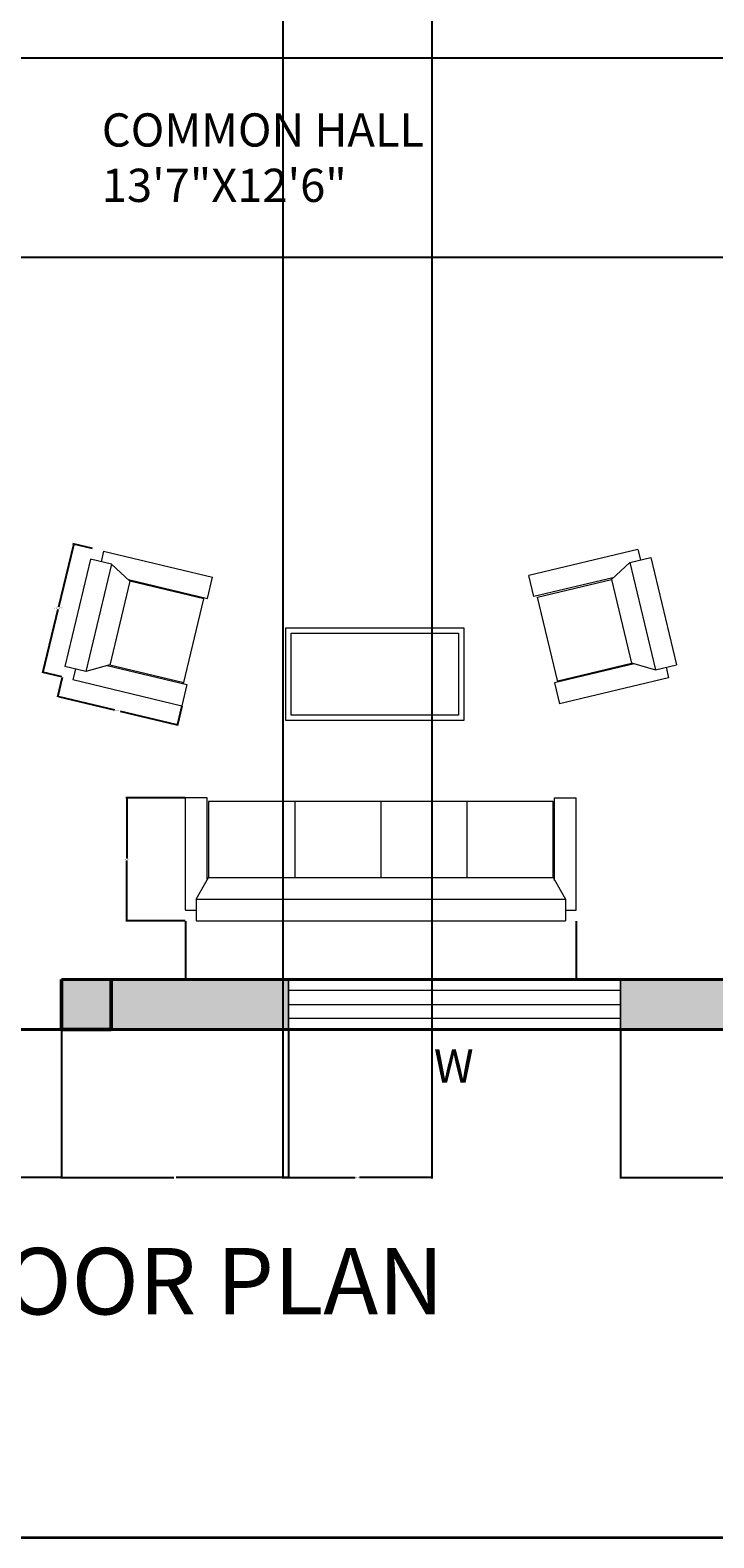
# Model space of a CAD drawing. Units: inches. Extents: x 25176543 to 25177243, y 80295576 to 80296086.
# Tile 5 of 11: x 25176879 to 25177002, y 80295576 to 80295848. Entities that reach past the tile are written whole.
import ezdxf

# ---------------------------------------------------------------- set-up
doc = ezdxf.new("R2010")
doc.units = ezdxf.units.IN
doc.header["$MEASUREMENT"] = 0
for name, color, linetype, lineweight in [('A-ANNO-DIMS', 2, 'Continuous', 18), ('A-ANNO-IDEN', 7, 'Continuous', 18), ('A-ANNO-TTLB', 7, 'Continuous', 35), ('A-AREA-IDEN', 7, 'Continuous', 18), ('A-COLS', 7, 'Continuous', 50), ('A-COLS-PATT', 251, 'Continuous', 13), ('A-GLAZ', 4, 'Continuous', 18), ('A-WALL', 7, 'Continuous', 40), ('A-WALL-PATT', 146, 'Continuous', 13), ('furniture', 31, 'Continuous', 13)]:
    doc.layers.add(name, color=color, linetype=linetype, lineweight=lineweight)
doc.styles.get("Standard").update_dxf_attribs({"font": 'arial.ttf'})
doc.dimstyles.get("Standard").update_dxf_attribs({"dimtxt": 0.18, "dimasz": 0.18, "dimexe": 0.18, "dimexo": 0.0625, "dimgap": 0.09, "dimtad": 0, "dimtih": 1, "dimtoh": 1, "dimdec": 4, "dimzin": 0, "dimdsep": 46, "dimtxsty": 'Standard', "dimcen": 0.09, "dimadec": 0, "dimazin": 0, "dimtfac": 1, "dimtdec": 4, "dimtofl": 0, "dimtmove": 0, "dimatfit": 3, "dimfxl": 1, "dimtolj": 1, "dimtzin": 0, "dimarcsym": 0})

# ---------------------------------------------------------------- blocks, each defined once
blk = doc.blocks.new('SOFA-FOUR-SEAT')
for p, q in [((0, 68.65), (0, 1.96)), ((3.92, 68.65), (0, 68.65)), ((1.96, 70.61), (22.23, 70.61)), ((1.96, 70.61), (1.96, 68.65)), ((3.92, 68.65), (3.92, 1.96)), ((3.92, 68.65), (7.85, 66.44)), ((22.23, 66.69), (22.23, 70.61)), ((7.54, 66.69), (22.23, 66.69)), ((21.58, 50.87), (7.85, 50.87)), ((21.58, 35.31), (7.85, 35.31)), ((21.58, 19.74), (7.85, 19.74)), ((7.85, 4.17), (3.92, 1.96)), ((7.29, 3.92), (22.23, 3.92)), ((22.23, 3.92), (22.23, 0)), ((3.92, 1.96), (0, 1.96)), ((1.96, 1.96), (1.96, 0)), ((1.96, 0), (22.23, 0))]:
    blk.add_line(p, q)
blk.add_lwpolyline([(7.85, 66.44), (7.85, 4.17), (21.58, 4.17), (21.58, 66.44)], close=True)
blk = doc.blocks.new('LOUNGE-CHAIR')
for p, q in [((0, 1.96), (0, 22.23)), ((3.92, 22.23), (0, 22.23)), ((3.92, 7.54), (3.92, 22.23)), ((19.93, 7.41), (19.93, 22.23)), ((19.93, 22.23), (23.85, 22.23)), ((23.85, 1.96), (23.85, 22.23)), ((19.74, 21.58), (19.74, 7.85)), ((1.96, 3.92), (4.17, 7.85)), ((19.68, 7.85), (21.89, 3.92)), ((1.96, 3.92), (21.89, 3.92)), ((1.96, 3.92), (1.96, 0)), ((21.89, 3.92), (21.89, 0)), ((0, 1.96), (1.96, 1.96)), ((1.96, 0), (21.89, 0)), ((21.89, 1.96), (23.85, 1.96))]:
    blk.add_line(p, q)
blk.add_lwpolyline([(19.93, 21.58), (4.17, 21.58), (4.17, 7.85), (19.74, 7.85)])
blk = doc.blocks.new('WIN-60IN')
for p, q in [((0, 9), (0, 0)), ((60, 9), (0, 9)), ((0, 9), (0, 4.5)), ((60, 0), (60, 9)), ((60, 7), (0, 7)), ((0, 4.5), (60, 4.5)), ((0, 2), (60, 2)), ((0, 0), (60, 0))]:
    blk.add_line(p, q)
blk = doc.blocks.new('*D26')
at = {"layer": 'A-ANNO-DIMS', "color": 0, "lineweight": -2, "transparency": 16777216}
for p, q in [((25176886.47, 80295755.29), (25176883.78, 80295744.06)), ((25176889.93, 80295754.65), (25176886.34, 80295755.51)), ((25176881.01, 80295732.45), (25176883.7, 80295743.69)), ((25176884.38, 80295731.46), (25176880.79, 80295732.32))]:
    blk.add_line(p, q, dxfattribs=at)
at = {"layer": 'A-ANNO-DIMS', "color": 0, "transparency": 16777216}
for points in [[(25176886.44, 80295755.3), (25176886.5, 80295755.29), (25176886.51, 80295755.47)], [(25176880.98, 80295732.46), (25176881.04, 80295732.44), (25176880.97, 80295732.27)]]:
    blk.add_solid(points, dxfattribs=at)
at = {"layer": 'Defpoints', "color": 0, "transparency": 16777216}
for p in [(25176889.99, 80295754.64), (25176880.97, 80295732.27), (25176884.45, 80295731.44)]:
    blk.add_point(p, dxfattribs=at)
at = {"layer": 'A-ANNO-DIMS', "color": 0, "transparency": 16777216, "insert": (25176883.74, 80295743.87), "char_height": 0.18, "attachment_point": 5}
blk.add_mtext('\\A1;CHAIR 24 TYP.', dxfattribs=at)
blk = doc.blocks.new('*D27')
at = {"layer": 'A-ANNO-DIMS', "color": 0, "lineweight": -2, "transparency": 16777216}
for p, q in [((25176884.43, 80295731.38), (25176883.57, 80295727.79)), ((25176883.79, 80295727.92), (25176893.89, 80295725.5)), ((25176906.05, 80295726.21), (25176905.19, 80295722.62)), ((25176905.06, 80295722.84), (25176894.95, 80295725.25))]:
    blk.add_line(p, q, dxfattribs=at)
at = {"layer": 'A-ANNO-DIMS', "color": 0, "transparency": 16777216}
for points in [[(25176883.8, 80295727.95), (25176883.78, 80295727.89), (25176883.61, 80295727.96)], [(25176905.07, 80295722.86), (25176905.05, 80295722.81), (25176905.23, 80295722.79)]]:
    blk.add_solid(points, dxfattribs=at)
at = {"layer": 'Defpoints', "color": 0, "transparency": 16777216}
for p in [(25176884.45, 80295731.44), (25176906.07, 80295726.27), (25176905.23, 80295722.79)]:
    blk.add_point(p, dxfattribs=at)
at = {"layer": 'A-ANNO-DIMS', "color": 0, "transparency": 16777216, "insert": (25176894.42, 80295725.38), "char_height": 0.18, "attachment_point": 5}
blk.add_mtext('\\A1;22 TYP.', dxfattribs=at)
blk = doc.blocks.new('*D30')
at = {"layer": 'A-ANNO-DIMS', "color": 0, "lineweight": -2, "transparency": 16777216}
for p, q in [((25176906.7, 80295687.32), (25176906.7, 80295676.61)), ((25176977.31, 80295687.32), (25176977.31, 80295676.61)), ((25176906.88, 80295676.79), (25176941.1, 80295676.79)), ((25176977.13, 80295676.79), (25176942.91, 80295676.79))]:
    blk.add_line(p, q, dxfattribs=at)
at = {"layer": 'A-ANNO-DIMS', "color": 0, "transparency": 16777216}
for points in [[(25176906.88, 80295676.82), (25176906.88, 80295676.76), (25176906.7, 80295676.79)], [(25176977.13, 80295676.82), (25176977.13, 80295676.76), (25176977.31, 80295676.79)]]:
    blk.add_solid(points, dxfattribs=at)
at = {"layer": 'Defpoints', "color": 0, "transparency": 16777216}
for p in [(25176906.7, 80295687.38), (25176977.31, 80295687.38), (25176906.7, 80295676.79)]:
    blk.add_point(p, dxfattribs=at)
at = {"layer": 'A-ANNO-DIMS', "color": 0, "transparency": 16777216, "insert": (25176942, 80295676.79), "char_height": 0.18, "attachment_point": 5}
blk.add_mtext('\\A1;SOFA 71 TYP.', dxfattribs=at)
blk = doc.blocks.new('*D31')
at = {"layer": 'A-ANNO-DIMS', "color": 0, "lineweight": -2, "transparency": 16777216}
for p, q in [((25176906.63, 80295709.61), (25176895.93, 80295709.61)), ((25176896.11, 80295709.43), (25176896.11, 80295698.67)), ((25176896.11, 80295687.56), (25176896.11, 80295698.31)), ((25176906.63, 80295687.38), (25176895.93, 80295687.38))]:
    blk.add_line(p, q, dxfattribs=at)
at = {"layer": 'A-ANNO-DIMS', "color": 0, "transparency": 16777216}
for points in [[(25176896.08, 80295709.43), (25176896.14, 80295709.43), (25176896.11, 80295709.61)], [(25176896.08, 80295687.56), (25176896.14, 80295687.56), (25176896.11, 80295687.38)]]:
    blk.add_solid(points, dxfattribs=at)
at = {"layer": 'Defpoints', "color": 0, "transparency": 16777216}
for p in [(25176896.11, 80295709.61), (25176906.7, 80295709.61), (25176906.7, 80295687.38)]:
    blk.add_point(p, dxfattribs=at)
at = {"layer": 'A-ANNO-DIMS', "color": 0, "transparency": 16777216, "insert": (25176896.11, 80295698.49), "char_height": 0.18, "attachment_point": 5}
blk.add_mtext('\\A1;22 TYP.', dxfattribs=at)
blk = doc.blocks.new('*D52')
at = {"layer": 'A-ANNO-DIMS', "color": 0, "lineweight": -2, "transparency": 16777216}
for p, q in [((25176842.3, 80295667.74), (25176842.3, 80295640.87)), ((25176884.3, 80295667.74), (25176884.3, 80295640.87)), ((25176842.48, 80295641.05), (25176863.08, 80295641.05)), ((25176884.12, 80295641.05), (25176863.52, 80295641.05))]:
    blk.add_line(p, q, dxfattribs=at)
at = {"layer": 'A-ANNO-DIMS', "color": 0, "transparency": 16777216}
for points in [[(25176842.48, 80295641.08), (25176842.48, 80295641.02), (25176842.3, 80295641.05)], [(25176884.12, 80295641.08), (25176884.12, 80295641.02), (25176884.3, 80295641.05)]]:
    blk.add_solid(points, dxfattribs=at)
at = {"layer": 'Defpoints', "color": 0, "transparency": 16777216}
for p in [(25176842.3, 80295667.8), (25176884.3, 80295667.8), (25176884.3, 80295641.05)]:
    blk.add_point(p, dxfattribs=at)
at = {"layer": 'A-ANNO-DIMS', "color": 0, "transparency": 16777216, "insert": (25176863.3, 80295641.05), "char_height": 0.18, "attachment_point": 5}
blk.add_mtext('\\A1;42', dxfattribs=at)
blk = doc.blocks.new('*D55')
at = {"layer": 'A-ANNO-DIMS', "color": 0, "lineweight": -2, "transparency": 16777216}
for p, q in [((25176884.3, 80295667.74), (25176884.3, 80295640.87)), ((25176925.3, 80295667.74), (25176925.3, 80295640.87)), ((25176884.48, 80295641.05), (25176904.6, 80295641.05)), ((25176925.12, 80295641.05), (25176905.01, 80295641.05))]:
    blk.add_line(p, q, dxfattribs=at)
at = {"layer": 'A-ANNO-DIMS', "color": 0, "transparency": 16777216}
for points in [[(25176884.48, 80295641.08), (25176884.48, 80295641.02), (25176884.3, 80295641.05)], [(25176925.12, 80295641.08), (25176925.12, 80295641.02), (25176925.3, 80295641.05)]]:
    blk.add_solid(points, dxfattribs=at)
at = {"layer": 'Defpoints', "color": 0, "transparency": 16777216}
for p in [(25176884.3, 80295667.8), (25176925.3, 80295667.8), (25176925.3, 80295641.05)]:
    blk.add_point(p, dxfattribs=at)
at = {"layer": 'A-ANNO-DIMS', "color": 0, "transparency": 16777216, "insert": (25176904.8, 80295641.05), "char_height": 0.18, "attachment_point": 5}
blk.add_mtext('\\A1;41', dxfattribs=at)
blk = doc.blocks.new('*D56')
at = {"layer": 'A-ANNO-DIMS', "color": 0, "lineweight": -2, "transparency": 16777216}
for p, q in [((25176985.3, 80295667.74), (25176985.3, 80295640.87)), ((25177030.59, 80295667.74), (25177030.59, 80295640.87)), ((25176985.48, 80295641.05), (25177007.55, 80295641.05)), ((25177030.41, 80295641.05), (25177008.34, 80295641.05))]:
    blk.add_line(p, q, dxfattribs=at)
at = {"layer": 'A-ANNO-DIMS', "color": 0, "transparency": 16777216}
for points in [[(25176985.48, 80295641.08), (25176985.48, 80295641.02), (25176985.3, 80295641.05)], [(25177030.41, 80295641.08), (25177030.41, 80295641.02), (25177030.59, 80295641.05)]]:
    blk.add_solid(points, dxfattribs=at)
at = {"layer": 'Defpoints', "color": 0, "transparency": 16777216}
for p in [(25176985.3, 80295667.8), (25177030.59, 80295667.8), (25177030.59, 80295641.05)]:
    blk.add_point(p, dxfattribs=at)
at = {"layer": 'A-ANNO-DIMS', "color": 0, "transparency": 16777216, "insert": (25177007.94, 80295641.05), "char_height": 0.18, "attachment_point": 5}
blk.add_mtext('\\A1;45.29', dxfattribs=at)
blk = doc.blocks.new('*D69')
at = {"layer": 'A-ANNO-DIMS', "color": 0, "lineweight": -2, "transparency": 16777216}
for p, q in [((25176924.3, 80295890.24), (25176924.3, 80295640.87)), ((25176951.22, 80295890.24), (25176951.22, 80295640.87)), ((25176924.48, 80295641.05), (25176937.37, 80295641.05)), ((25176951.04, 80295641.05), (25176938.16, 80295641.05))]:
    blk.add_line(p, q, dxfattribs=at)
at = {"layer": 'A-ANNO-DIMS', "color": 0, "transparency": 16777216}
for points in [[(25176924.48, 80295641.08), (25176924.48, 80295641.02), (25176924.3, 80295641.05)], [(25176951.04, 80295641.08), (25176951.04, 80295641.02), (25176951.22, 80295641.05)]]:
    blk.add_solid(points, dxfattribs=at)
at = {"layer": 'Defpoints', "color": 0, "transparency": 16777216}
for p in [(25176924.3, 80295890.3), (25176951.22, 80295890.3), (25176951.22, 80295641.05)]:
    blk.add_point(p, dxfattribs=at)
at = {"layer": 'A-ANNO-DIMS', "color": 0, "transparency": 16777216, "insert": (25176937.76, 80295641.05), "char_height": 0.18, "attachment_point": 5}
blk.add_mtext('\\A1;26.92', dxfattribs=at)
blk = doc.blocks.new('*D73')
at = {"layer": 'A-ANNO-DIMS', "color": 0, "lineweight": -2, "transparency": 16777216}
for p, q in [((25176791.86, 80295843.3), (25177152.73, 80295843.3)), ((25177152.55, 80295843.12), (25177152.55, 80295825.48)), ((25177152.55, 80295807.48), (25177152.55, 80295825.12)), ((25176791.86, 80295807.3), (25177152.73, 80295807.3))]:
    blk.add_line(p, q, dxfattribs=at)
at = {"layer": 'A-ANNO-DIMS', "color": 0, "transparency": 16777216}
for points in [[(25177152.52, 80295843.12), (25177152.58, 80295843.12), (25177152.55, 80295843.3)], [(25177152.52, 80295807.48), (25177152.58, 80295807.48), (25177152.55, 80295807.3)]]:
    blk.add_solid(points, dxfattribs=at)
at = {"layer": 'Defpoints', "color": 0, "transparency": 16777216}
for p in [(25176791.8, 80295843.3), (25177152.55, 80295843.3), (25176791.8, 80295807.3)]:
    blk.add_point(p, dxfattribs=at)
at = {"layer": 'A-ANNO-DIMS', "color": 0, "transparency": 16777216, "insert": (25177152.55, 80295825.3), "char_height": 0.18, "attachment_point": 5}
blk.add_mtext('\\A1;36', dxfattribs=at)

msp = doc.modelspace()

# ---------------------------------------------------------------- hatches: boundary and pattern name
at = {"layer": 'A-COLS-PATT'}
h = msp.add_hatch(color=256, dxfattribs=at)
h.dxf.hatch_style = 1
h.paths.add_polyline_path([(25176658.8016, 80296025.3022), (25176649.8016, 80296025.3022), (25176649.8016, 80296016.3022), (25176658.8016, 80296016.3022)])
h.paths.add_polyline_path([(25176819.3016, 80296025.3022), (25176810.3016, 80296025.3022), (25176810.3016, 80296016.3022), (25176819.3016, 80296016.3022)])
h.paths.add_polyline_path([(25176876.3016, 80296025.3022), (25176867.3016, 80296025.3022), (25176867.3016, 80296016.3022), (25176876.3016, 80296016.3022)])
h.paths.add_polyline_path([(25177013.3016, 80296025.3022), (25177004.3016, 80296025.3022), (25177004.3016, 80296016.3022), (25177013.3016, 80296016.3022)])
h.paths.add_polyline_path([(25176819.3016, 80295890.3022), (25176810.3016, 80295890.3022), (25176810.3016, 80295881.3022), (25176819.3016, 80295881.3022)])
h.paths.add_polyline_path([(25176658.8016, 80295890.3022), (25176649.8016, 80295890.3022), (25176649.8016, 80295881.3022), (25176658.8016, 80295881.3022)])
h.paths.add_polyline_path([(25177125.8016, 80296025.3022), (25177116.8016, 80296025.3022), (25177116.8016, 80296016.3022), (25177125.8016, 80296016.3022)])
h.paths.add_polyline_path([(25177125.8016, 80295848.3022), (25177116.8016, 80295848.3022), (25177116.8016, 80295839.3022), (25177125.8016, 80295839.3022)])
h.paths.add_polyline_path([(25177013.3016, 80295848.3022), (25177004.3016, 80295848.3022), (25177004.3016, 80295839.3022), (25177013.3016, 80295839.3022)])
h.paths.add_polyline_path([(25177125.8016, 80295676.8022), (25177116.8016, 80295676.8022), (25177116.8016, 80295667.8022), (25177125.8016, 80295667.8022)])
h.paths.add_polyline_path([(25177013.3016, 80295676.8022), (25177004.3016, 80295676.8022), (25177004.3016, 80295667.8022), (25177013.3016, 80295667.8022)])
h.paths.add_polyline_path([(25176842.3016, 80295676.8022), (25176833.3016, 80295676.8022), (25176833.3016, 80295667.8022), (25176842.3016, 80295667.8022)])
h.paths.add_polyline_path([(25176893.3016, 80295676.8022), (25176884.3016, 80295676.8022), (25176884.3016, 80295667.8022), (25176893.3016, 80295667.8022)])
h.paths.add_polyline_path([(25176842.3016, 80295807.3022), (25176833.3016, 80295807.3022), (25176833.3016, 80295798.3022), (25176842.3016, 80295798.3022)])
h.paths.add_polyline_path([(25176658.8016, 80295807.3022), (25176649.8016, 80295807.3022), (25176649.8016, 80295798.3022), (25176658.8016, 80295798.3022)])
h.paths.add_polyline_path([(25176658.8016, 80295676.8022), (25176649.8016, 80295676.8022), (25176649.8016, 80295667.8022), (25176658.8016, 80295667.8022)])
at = {"layer": 'A-WALL-PATT'}
h = msp.add_hatch(color=256, dxfattribs=at)
h.dxf.hatch_style = 1
h.paths.add_polyline_path([(25176705.5738, 80295676.8022), (25176658.8016, 80295676.8022), (25176658.8016, 80295667.8022), (25176705.5738, 80295667.8022)])
h.paths.add_polyline_path([(25176833.3016, 80295676.8022), (25176765.5738, 80295676.8022), (25176765.5738, 80295667.8022), (25176833.3016, 80295667.8022)])
h.paths.add_polyline_path([(25176925.2997, 80295676.8022), (25176893.3016, 80295676.8022), (25176893.3016, 80295667.8022), (25176925.2997, 80295667.8022)])
h.paths.add_polyline_path([(25177004.3016, 80295676.8022), (25176985.2997, 80295676.8022), (25176985.2997, 80295667.8022), (25177004.3016, 80295667.8022)])
h.paths.add_polyline_path([(25177030.5901, 80295676.8022), (25177013.3016, 80295676.8022), (25177013.3016, 80295667.8022), (25177030.5901, 80295667.8022)])
h.paths.add_polyline_path([(25177116.8016, 80295676.8022), (25177090.5901, 80295676.8022), (25177090.5901, 80295667.8022), (25177116.8016, 80295667.8022)])
h.paths.add_polyline_path([(25177125.8016, 80295729.6384), (25177116.8016, 80295729.6384), (25177116.8016, 80295676.8022), (25177125.8016, 80295676.8022)])
h.paths.add_polyline_path([(25177125.8016, 80295839.3022), (25177116.8016, 80295839.3022), (25177116.8016, 80295789.6384), (25177121.3016, 80295789.6384), (25177125.8016, 80295789.6384)])

# ---------------------------------------------------------------- linework, layer by layer
at = {"layer": 'A-ANNO-TTLB'}
msp.add_lwpolyline([(25176542.8973, 80296086.2335), (25177242.9194, 80296086.2335), (25177242.9194, 80295575.9501), (25176542.8973, 80295575.9501)], close=True, dxfattribs=at)
at = {"layer": 'A-COLS'}
for p, q in [((25176884.3016, 80295667.8022), (25176884.3016, 80295676.8022)), ((25176893.3016, 80295667.8022), (25176893.3016, 80295676.8022)), ((25176884.3016, 80295667.8022), (25176893.3016, 80295667.8022))]:
    msp.add_line(p, q, dxfattribs=at)
at = {"layer": 'A-GLAZ'}
for p, q in [((25176925.2997, 80295667.8022), (25176925.2997, 80295676.8022)), ((25176985.2997, 80295676.8022), (25176985.2997, 80295667.8022)), ((25176985.2997, 80295667.8022), (25176925.2997, 80295667.8022))]:
    msp.add_line(p, q, dxfattribs=at)
at = {"layer": 'A-WALL'}
for p, q in [((25176884.3016, 80295676.8022), (25177125.8016, 80295676.8022)), ((25176649.8016, 80295667.8022), (25177125.8016, 80295667.8022)), ((25176878.3016, 80295667.8022), (25176884.3016, 80295667.8022))]:
    msp.add_line(p, q, dxfattribs=at)
at = {"layer": 'furniture'}
for points in [[(25176924.8328, 80295740.3649), (25176957.0172, 80295740.3649), (25176957.0172, 80295723.5811), (25176924.8328, 80295723.5811)], [(25176925.8328, 80295739.3649), (25176956.0172, 80295739.3649), (25176956.0172, 80295724.5811), (25176925.8328, 80295724.5811)]]:
    msp.add_lwpolyline(points, close=True, dxfattribs=at)

# ---------------------------------------------------------------- block references
at = {"layer": 'A-GLAZ'}
msp.add_blockref('WIN-60IN', (25176925.2996, 80295667.802), dxfattribs=at)
at = {"layer": 'furniture'}
for name, p, rotation in [('LOUNGE-CHAIR', (25176889.9919, 80295754.6374), 256.5521747299599), ('SOFA-FOUR-SEAT', (25176977.3072, 80295687.3788), 89.99999999822946)]:
    msp.add_blockref(name, p, dxfattribs=dict(at, rotation=rotation))
at = {"layer": 'furniture', "extrusion": (0, 0, -1), "zscale": -1, "rotation": 256.552174564094}
msp.add_blockref('LOUNGE-CHAIR', (-25176990.3644, 80295754.9575), dxfattribs=at)

# ---------------------------------------------------------------- texts
at = {"layer": 'A-ANNO-IDEN', "insert": (25176951.596, 80295664.1768), "char_height": 6, "attachment_point": 1}
msp.add_mtext_dynamic_manual_height_columns('W', width=24.139595, gutter_width=1, heights=[0], dxfattribs=at)
at = {"layer": 'A-ANNO-TTLB', "insert": (25176783.6607, 80295628.3104), "char_height": 12, "attachment_point": 1}
msp.add_mtext_dynamic_manual_height_columns('GROUND FLOOR PLAN', width=295.824021, gutter_width=1, heights=[0], dxfattribs=at)
at = {"layer": 'A-AREA-IDEN', "insert": (25176891.5888, 80295833.2732), "char_height": 6, "attachment_point": 1}
msp.add_mtext_dynamic_manual_height_columns('COMMON HALL\\P13\'7"X12\'6"', width=80.848097, gutter_width=1, heights=[0], dxfattribs=at)

# ---------------------------------------------------------------- dimensions: what is measured, and where the dimension line sits
at = {"layer": 'A-ANNO-DIMS'}
for base, p1, p2, override, picture, middle in [((25176951.2221, 80295641.0522), (25176924.3016, 80295890.3022), (25176951.2221, 80295890.3022), {"dimdec": 2, "dimlfac": 1, "dimrnd": 0, "dimzin": 0, "dimdsep": 46, "dimlunit": 2}, '*D69', (25176937.7618, 80295641.0522)), ((25176884.3016, 80295641.0522), (25176842.3016, 80295667.8022), (25176884.3016, 80295667.8022), {"dimdec": 0, "dimlfac": 1, "dimrnd": 0, "dimzin": 0, "dimdsep": 46, "dimlunit": 2}, '*D52', (25176863.3016, 80295641.0522)), ((25176925.2997, 80295641.0522), (25176884.3016, 80295667.8022), (25176925.2997, 80295667.8022), {"dimdec": 0, "dimlfac": 1, "dimrnd": 0, "dimzin": 0, "dimdsep": 46, "dimlunit": 2}, '*D55', (25176904.8006, 80295641.0522)), ((25177030.5901, 80295641.0522), (25176985.2997, 80295667.8022), (25177030.5901, 80295667.8022), {"dimdec": 2, "dimlfac": 1, "dimrnd": 0, "dimzin": 0, "dimdsep": 46, "dimlunit": 2}, '*D56', (25177007.9449, 80295641.0522))]:
    dim = msp.add_linear_dim(base=base, p1=p1, p2=p2, dimstyle='Standard', override=override, dxfattribs=at)
    dim.commit()
    dim.dimension.update_dxf_attribs({"geometry": picture, "text_midpoint": middle})
dim = msp.add_linear_dim(base=(25177152.5516, 80295843.3022), p1=(25176791.8016, 80295807.3022), p2=(25176791.8016, 80295843.3022), angle=90, dimstyle='Standard', override={"dimdec": 0, "dimlfac": 1, "dimrnd": 0, "dimzin": 0, "dimdsep": 46, "dimlunit": 2}, dxfattribs=at)
dim.commit()
dim.dimension.update_dxf_attribs({"geometry": '*D73', "text_midpoint": (25177152.5516, 80295825.3022)})
for base, p1, p2, angle, text, picture, middle in [((25176880.9664, 80295732.2743), (25176889.9921, 80295754.6377), (25176884.4457, 80295731.4424), 256.552175, 'CHAIR <> TYP.', '*D26', (25176883.7396, 80295743.872)), ((25176905.2333, 80295722.7935), (25176884.4457, 80295731.4424), (25176906.0652, 80295726.2728), 346.552175, '<> TYP.', '*D27', (25176894.4235, 80295725.3783)), ((25176896.1056, 80295709.6083), (25176906.6971, 80295687.3793), (25176906.6971, 80295709.6083), 90, '<> TYP.', '*D31', (25176896.1056, 80295698.4938)), ((25176906.6971, 80295676.7878), (25176977.3069, 80295687.3793), (25176906.6971, 80295687.3793), 180, 'SOFA <> TYP.', '*D30', (25176942.002, 80295676.7878))]:
    dim = msp.add_linear_dim(base=base, p1=p1, p2=p2, angle=angle, text=text, dimstyle='Standard', override={"dimdec": 0, "dimlfac": 1, "dimrnd": 0, "dimzin": 0, "dimdsep": 46, "dimlunit": 2}, dxfattribs=at)
    dim.commit()
    dim.dimension.update_dxf_attribs({"geometry": picture, "text_midpoint": middle})

doc.saveas('drawing.dxf')
